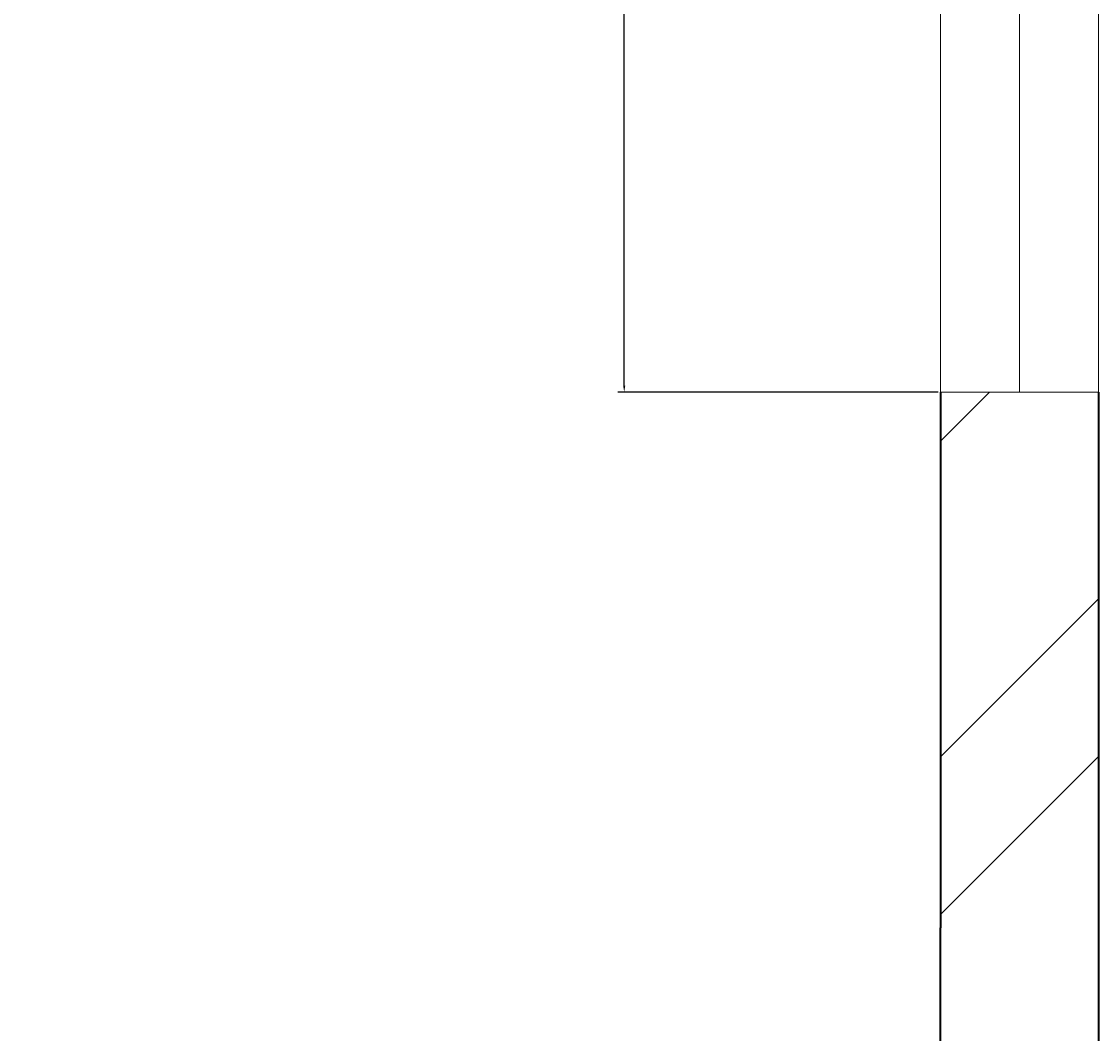
# Model space of a CAD drawing. Units: inches. Extents: x 1885 to 2748, y 783 to 2421.
# Tile 103 of 117: x 2588 to 2618, y 1879 to 1907. Entities that reach past the tile are written whole.
import ezdxf

# ---------------------------------------------------------------- set-up
doc = ezdxf.new("R2010")
doc.units = ezdxf.units.IN
for name, color, linetype, lineweight in [('A-ANNO-DIMS', 2, 'Continuous', 18), ('A-GLAZ', 181, 'Continuous', 18), ('A-WALL', 7, 'Continuous', 35)]:
    doc.layers.add(name, color=color, linetype=linetype, lineweight=lineweight)
doc.layers.add('A-WALL-PATT', color=85, linetype='Continuous', lineweight=13, true_color=0x58ba48)
doc.styles.get("Standard").update_dxf_attribs({"font": 'arial.ttf'})
doc.dimstyles.get("Standard").update_dxf_attribs({"dimtxt": 0.18, "dimasz": 0.18, "dimexe": 0.18, "dimexo": 0.0625, "dimgap": 0.09, "dimtad": 0, "dimtih": 1, "dimtoh": 1, "dimdec": 4, "dimzin": 0, "dimdsep": 46, "dimtxsty": 'Standard', "dimcen": 0.09, "dimadec": 0, "dimazin": 0, "dimtfac": 1, "dimtdec": 4, "dimtofl": 0, "dimtmove": 0, "dimatfit": 3, "dimfxl": 1, "dimtolj": 1, "dimtzin": 0, "dimarcsym": 0})

# ---------------------------------------------------------------- blocks, each defined once
blk = doc.blocks.new('WIN-60-ALT')
for p, q in [((0.004, 59.998), (0.004, -0.002)), ((2.254, 59.998), (2.254, -0.002)), ((4.504, -0.002), (4.504, 59.998)), ((4.504, -0.002), (0.004, -0.002)), ((2.254, -0.002), (4.504, -0.002))]:
    blk.add_line(p, q)
blk = doc.blocks.new('*D17')
at = {"layer": 'A-ANNO-DIMS', "color": 0, "lineweight": -2, "transparency": 16777216}
for p, q in [((2613.711, 1956.755), (2604.594, 1956.755)), ((2604.774, 1956.575), (2604.774, 1926.938)), ((2604.774, 1896.935), (2604.774, 1926.572)), ((2613.711, 1896.755), (2604.594, 1896.755))]:
    blk.add_line(p, q, dxfattribs=at)
at = {"layer": 'A-ANNO-DIMS', "color": 0, "transparency": 16777216}
for points in [[(2604.744, 1956.575), (2604.804, 1956.575), (2604.774, 1956.755)], [(2604.744, 1896.935), (2604.804, 1896.935), (2604.774, 1896.755)]]:
    blk.add_solid(points, dxfattribs=at)
at = {"layer": 'Defpoints', "color": 0, "transparency": 16777216}
for p in [(2604.774, 1956.755), (2613.774, 1956.755), (2613.774, 1896.755)]:
    blk.add_point(p, dxfattribs=at)
at = {"layer": 'A-ANNO-DIMS', "color": 0, "transparency": 16777216, "insert": (2604.774, 1926.755), "char_height": 0.18, "attachment_point": 5}
blk.add_mtext('\\A1;ALT. WINDOW 60 TYP.', dxfattribs=at)

msp = doc.modelspace()

# ---------------------------------------------------------------- hatches: boundary and pattern name
at = {"layer": 'A-WALL-PATT'}
h = msp.add_hatch(dxfattribs=at)
h.set_pattern_fill('ANSI32', color=256)
h.paths.add_polyline_path([(2007.772, 2318.006), (1980.774, 2318.006), (1980.774, 2281.215), (1985.274, 2281.215), (1985.274, 2313.506), (2007.772, 2313.506), (2007.772, 2315.756)])
h.paths.add_polyline_path([(2094.324, 2318.006), (2067.772, 2318.006), (2067.772, 2313.506), (2094.324, 2313.506), (2094.324, 2315.756)])
h.paths.add_polyline_path([(2131.367, 2315.756), (2131.367, 2318.006), (2131.189, 2318.006), (2112.609, 2318.006), (2112.609, 2313.506), (2117.274, 2313.506), (2117.274, 2255.201), (2121.774, 2255.201), (2121.774, 2313.506), (2131.367, 2313.506)])
h.paths.add_polyline_path([(2190.512, 2318.006), (2155.367, 2318.006), (2155.367, 2313.506), (2169.774, 2313.506), (2169.774, 2229.506), (2121.774, 2229.506), (2121.774, 2233.451), (2119.524, 2233.451), (2117.274, 2233.451), (2117.274, 2201.101), (2121.774, 2201.101), (2121.774, 2225.006), (2169.774, 2225.006), (2169.774, 2165.006), (2306.274, 2165.006), (2306.274, 2066.006), (2310.774, 2066.006), (2344.274, 2066.006), (2486.274, 2066.006), (2486.274, 1886.006), (2483.02, 1886.006), (2483.02, 1881.506), (2486.274, 1881.506), (2486.274, 1880.678), (2490.774, 1880.678), (2490.774, 2070.506), (2344.274, 2070.506), (2310.774, 2070.506), (2310.774, 2165.006), (2310.774, 2173.636), (2308.524, 2173.636), (2306.274, 2173.636), (2306.274, 2169.506), (2174.274, 2169.506), (2174.274, 2313.506), (2190.512, 2313.506), (2190.512, 2315.756)])
h.paths.add_polyline_path([(1985.274, 2221.215), (1980.774, 2221.215), (1980.774, 2165.006), (1992.774, 2165.006), (1992.774, 2141.927), (1997.274, 2141.927), (1997.274, 2165.006), (2117.274, 2165.006), (2117.274, 2163.126), (2121.774, 2163.126), (2121.774, 2172.734), (2119.524, 2172.734), (2117.274, 2172.734), (2117.274, 2169.506), (1985.274, 2169.506)])
h.paths.add_polyline_path([(1997.274, 2105.927), (1992.774, 2105.927), (1992.774, 2070.506), (2016.774, 2070.506), (2016.774, 2059.123), (2019.024, 2059.123), (2021.274, 2059.123), (2021.274, 2070.506), (2117.274, 2070.506), (2117.274, 2022.506), (2114.423, 2022.506), (2114.423, 2018.006), (2123.627, 2018.006), (2123.627, 2020.256), (2123.627, 2022.506), (2121.774, 2022.506), (2121.774, 2142.587), (2119.524, 2142.587), (2117.274, 2142.587), (2117.274, 2075.006), (1997.274, 2075.006)])
h.paths.add_polyline_path([(2092.029, 2020.256), (2092.029, 2022.506), (2021.274, 2022.506), (2021.274, 2035.123), (2016.774, 2035.123), (2016.774, 2018.006), (2016.774, 1978.784), (2021.274, 1978.784), (2021.274, 2018.006), (2092.029, 2018.006)])
h.paths.add_polyline_path([(2260.938, 2022.506), (2153.105, 2022.506), (2153.105, 2020.256), (2153.105, 2018.006), (2155.274, 2018.006), (2155.274, 1886.006), (2107.629, 1886.006), (2107.629, 1881.506), (2182.911, 1881.506), (2182.911, 1883.756), (2182.911, 1886.006), (2159.774, 1886.006), (2159.774, 2018.006), (2260.938, 2018.006), (2260.938, 2020.256)])
h.paths.add_polyline_path([(2047.629, 1883.756), (2047.629, 1886.006), (2021.274, 1886.006), (2021.274, 1918.784), (2019.024, 1918.784), (2016.774, 1918.784), (2016.774, 1881.506), (2047.629, 1881.506)])
h.paths.add_polyline_path([(2306.361, 1883.756), (2306.361, 1886.006), (2296.274, 1886.006), (2296.274, 1982.006), (2316.535, 1982.006), (2316.535, 1984.256), (2316.535, 1986.506), (2296.274, 1986.506), (2296.274, 2022.506), (2289.276, 2022.506), (2289.276, 2018.006), (2291.774, 2018.006), (2291.774, 1886.006), (2242.911, 1886.006), (2242.911, 1881.506), (2306.361, 1881.506)], flags=17)
h.paths.add_polyline_path([(1985.274, 1843.006), (2021.6, 1843.006), (2021.534, 1845.441), (2021.477, 1847.506), (1980.774, 1847.506), (1980.774, 1809.446), (1985.274, 1809.446)])
h.paths.add_polyline_path([(2131.482, 1845.256), (2131.482, 1847.506), (2081.534, 1847.506), (2081.534, 1843.006), (2117.274, 1843.006), (2117.274, 1784.147), (2119.524, 1784.147), (2121.774, 1784.147), (2121.774, 1843.006), (2131.482, 1843.006)])
h.paths.add_polyline_path([(2203.886, 1847.506), (2155.482, 1847.506), (2155.482, 1843.006), (2169.774, 1843.006), (2169.774, 1759.006), (2121.774, 1759.006), (2121.774, 1761.457), (2117.274, 1761.457), (2117.274, 1730.429), (2121.774, 1730.429), (2121.774, 1754.506), (2177.421, 1754.506), (2177.421, 1756.756), (2177.421, 1759.006), (2174.274, 1759.006), (2174.274, 1843.006), (2203.886, 1843.006)])
h.paths.add_polyline_path([(2335.554, 1845.256), (2335.554, 1847.506), (2239.886, 1847.506), (2239.886, 1843.006), (2306.274, 1843.006), (2306.274, 1759.006), (2199.486, 1759.006), (2199.486, 1754.506), (2310.774, 1754.506), (2310.774, 1843.006), (2335.554, 1843.006)])
h.paths.add_polyline_path([(2348.774, 2022.506), (2344.274, 2022.506), (2344.274, 1986.506), (2341.681, 1986.506), (2341.681, 1982.006), (2344.274, 1982.006), (2344.274, 1886.006), (2330.361, 1886.006), (2330.361, 1881.506), (2361.627, 1881.506), (2361.627, 1883.756), (2361.627, 1886.006), (2348.774, 1886.006)], flags=17)
h.paths.add_polyline_path([(2283.251, 2315.756), (2283.251, 2318.006), (2238.512, 2318.006), (2238.512, 2313.506), (2283.251, 2313.506)], flags=17)
h.paths.add_polyline_path([(2363.274, 2348.006), (2388.677, 2348.006), (2388.677, 2350.256), (2388.677, 2352.506), (2358.774, 2352.506), (2358.774, 2348.006), (2358.774, 2318.006), (2344.481, 2318.006), (2344.481, 2313.506), (2358.774, 2313.506), (2358.774, 2229.506), (2310.774, 2229.506), (2310.774, 2231.952), (2306.274, 2231.952), (2306.274, 2205.611), (2310.774, 2205.611), (2310.774, 2225.006), (2358.774, 2225.006), (2358.774, 2211.506), (2452.329, 2211.506), (2452.329, 2213.756), (2452.329, 2216.006), (2363.274, 2216.006), (2363.274, 2318.006)])
h.paths.add_polyline_path([(2310.774, 2313.506), (2320.481, 2313.506), (2320.481, 2315.756), (2320.481, 2318.006), (2302.728, 2318.006), (2302.728, 2313.506), (2306.274, 2313.506), (2306.274, 2251.076), (2310.774, 2251.076)], flags=17)
h.paths.add_polyline_path([(2490.774, 2352.506), (2486.274, 2352.506), (2448.677, 2352.506), (2448.677, 2348.006), (2486.274, 2348.006), (2486.274, 2318.006), (2486.274, 2216.006), (2481.78, 2216.006), (2481.78, 2211.506), (2486.274, 2211.506), (2486.274, 2165.006), (2493.289, 2165.006), (2493.289, 2167.256), (2493.289, 2169.506), (2490.774, 2169.506), (2490.774, 2313.506), (2494.429, 2313.506), (2494.429, 2318.006), (2490.774, 2318.006)])
h.paths.add_polyline_path([(2534.653, 2318.006), (2515.691, 2318.006), (2515.691, 2313.506), (2534.653, 2313.506), (2534.653, 2315.756)])
h.paths.add_polyline_path([(2618.274, 2318.006), (2594.653, 2318.006), (2594.653, 2313.506), (2613.774, 2313.506), (2613.774, 2281.706), (2618.274, 2281.706)])
h.paths.add_polyline_path([(2618.274, 2221.706), (2613.774, 2221.706), (2613.774, 2169.506), (2554.019, 2169.506), (2554.019, 2165.006), (2613.774, 2165.006), (2613.774, 2152.878), (2618.274, 2152.878)])
h.paths.add_polyline_path([(2618.274, 2128.878), (2616.024, 2128.878), (2613.774, 2128.878), (2613.774, 2117.006), (2529.774, 2117.006), (2529.774, 2165.006), (2532.848, 2165.006), (2532.848, 2169.506), (2522.867, 2169.506), (2522.867, 2165.006), (2525.274, 2165.006), (2525.274, 2117.006), (2525.274, 2112.506), (2525.274, 2108.576), (2529.774, 2108.576), (2529.774, 2112.506), (2613.774, 2112.506), (2613.774, 2080.19), (2618.274, 2080.19)])
h.paths.add_polyline_path([(2618.274, 2044.19), (2616.024, 2044.19), (2613.774, 2044.19), (2613.774, 2015.506), (2529.774, 2015.506), (2529.774, 2088.582), (2527.524, 2088.582), (2525.274, 2088.582), (2525.274, 2011.006), (2613.774, 2011.006), (2613.774, 1956.755), (2618.274, 1956.755)])
h.paths.add_polyline_path([(2618.274, 1881.506), (2618.274, 1896.755), (2613.774, 1896.755), (2613.774, 1881.506), (2613.774, 1847.506), (2592.715, 1847.506), (2592.715, 1843.006), (2613.774, 1843.006), (2613.774, 1765.006), (2613.774, 1760.506), (2609.621, 1760.506), (2609.621, 1756.006), (2613.774, 1756.006), (2613.774, 1660.006), (2608.544, 1660.006), (2608.544, 1655.506), (2613.774, 1655.506), (2613.774, 1508.158), (2618.274, 1508.158)])
h.paths.add_polyline_path([(2565.774, 1843.006), (2568.997, 1843.006), (2568.997, 1847.506), (2490.774, 1847.506), (2490.774, 1849.7), (2488.524, 1849.7), (2486.274, 1849.7), (2486.274, 1847.506), (2477.274, 1847.506), (2477.274, 1838.506), (2477.274, 1821.493), (2486.274, 1821.493), (2486.274, 1838.506), (2561.274, 1838.506), (2561.274, 1765.006), (2486.274, 1765.006), (2486.274, 1786.157), (2477.274, 1786.157), (2477.274, 1765.006), (2477.274, 1756.006), (2486.274, 1756.006), (2565.774, 1756.006), (2585.621, 1756.006), (2585.621, 1758.256), (2585.621, 1760.506), (2565.774, 1760.506), (2565.774, 1765.006)])
h.paths.add_polyline_path([(2486.274, 1651.006), (2561.274, 1651.006), (2561.274, 1567.006), (2486.274, 1567.006), (2486.274, 1591.321), (2477.274, 1591.321), (2477.274, 1567.006), (2477.274, 1558.006), (2477.274, 1555.439), (2481.774, 1555.439), (2481.774, 1558.006), (2568.653, 1558.006), (2568.653, 1560.256), (2568.653, 1562.506), (2565.774, 1562.506), (2565.774, 1655.506), (2584.544, 1655.506), (2584.544, 1657.756), (2584.544, 1660.006), (2565.774, 1660.006), (2486.274, 1660.006), (2477.274, 1660.006), (2477.274, 1651.006), (2477.274, 1632.989), (2486.274, 1632.989)])
h.paths.add_polyline_path([(2449.967, 1883.756), (2449.967, 1886.006), (2421.627, 1886.006), (2421.627, 1881.506), (2449.967, 1881.506)], flags=17)
h.paths.add_polyline_path([(2447.274, 1847.506), (2395.554, 1847.506), (2395.554, 1843.006), (2442.774, 1843.006), (2442.774, 1809.27), (2447.274, 1809.27)])
h.paths.add_polyline_path([(1985.274, 1749.446), (1980.774, 1749.446), (1980.774, 1694.504), (1985.274, 1694.504), (1985.274, 1694.506), (1986.897, 1694.506), (1986.897, 1697.78), (1986.897, 1699.006), (1985.274, 1699.006)])
h.paths.add_polyline_path([(2152.774, 1699.006), (2121.774, 1699.006), (2121.774, 1703.668), (2119.524, 1703.668), (2117.274, 1703.668), (2117.274, 1699.006), (2009.219, 1699.006), (2009.219, 1694.506), (2148.274, 1694.506), (2148.274, 1692.631), (2152.774, 1692.631)])
h.paths.add_polyline_path([(2016.274, 1694.506), (2011.774, 1694.506), (2011.774, 1558.006), (2040.806, 1558.006), (2040.806, 1560.256), (2040.806, 1562.506), (2016.274, 1562.506)])
h.paths.add_polyline_path([(2152.774, 1663.017), (2150.524, 1663.017), (2148.274, 1663.017), (2148.274, 1562.506), (2100.806, 1562.506), (2100.806, 1558.006), (2165.119, 1558.006), (2165.119, 1560.256), (2165.119, 1562.506), (2152.774, 1562.506), (2152.774, 1610.506), (2224.774, 1610.506), (2224.774, 1607.99), (2229.274, 1607.99), (2229.274, 1615.006), (2152.774, 1615.006)])
h.paths.add_polyline_path([(2238.613, 1560.256), (2238.613, 1562.506), (2229.274, 1562.506), (2229.274, 1588.756), (2227.024, 1588.763), (2224.774, 1588.771), (2224.774, 1562.506), (2189.119, 1562.506), (2189.119, 1558.006), (2238.613, 1558.006)])
h.paths.add_polyline_path([(2336.024, 1560.256), (2336.024, 1562.506), (2310.774, 1562.506), (2310.774, 1656.347), (2308.524, 1656.347), (2306.274, 1656.347), (2306.274, 1562.506), (2286.613, 1562.506), (2286.613, 1558.006), (2336.024, 1558.006)])
h.paths.add_polyline_path([(2447.274, 1690.968), (2445.024, 1690.968), (2442.774, 1690.968), (2442.774, 1687.006), (2306.274, 1687.006), (2306.274, 1680.75), (2310.774, 1680.75), (2310.774, 1682.506), (2442.774, 1682.506), (2442.774, 1562.506), (2396.024, 1562.506), (2396.024, 1558.006), (2447.274, 1558.006)])
h.paths.add_polyline_path([(2447.274, 1749.27), (2445.024, 1749.27), (2442.774, 1749.27), (2442.774, 1717.232), (2447.274, 1717.232)])
h.paths.add_polyline_path([(2044.674, 1521.756), (2044.674, 1524.006), (2007.274, 1524.006), (2007.274, 1503.49), (2009.524, 1503.49), (2011.774, 1503.49), (2011.774, 1519.506), (2044.674, 1519.506)])
h.paths.add_polyline_path([(2177.969, 1521.756), (2177.969, 1524.006), (2104.674, 1524.006), (2104.674, 1519.506), (2145.774, 1519.506), (2145.774, 1387.506), (2143.37, 1387.506), (2143.37, 1383.006), (2251.585, 1383.006), (2251.585, 1385.256), (2251.585, 1387.506), (2150.274, 1387.506), (2150.274, 1519.506), (2177.969, 1519.506)])
h.paths.add_polyline_path([(2298.704, 1524.006), (2237.969, 1524.006), (2237.969, 1519.506), (2282.274, 1519.506), (2282.274, 1387.506), (2279.683, 1387.506), (2279.683, 1383.006), (2286.774, 1383.006), (2286.774, 1419.006), (2312.451, 1419.006), (2312.451, 1421.256), (2312.451, 1423.506), (2286.774, 1423.506), (2286.774, 1519.506), (2298.704, 1519.506), (2298.704, 1521.722)], flags=17)
h.paths.add_polyline_path([(2361.897, 1521.756), (2361.897, 1524.006), (2322.704, 1524.006), (2322.704, 1519.506), (2334.774, 1519.506), (2334.774, 1423.506), (2331.93, 1423.506), (2331.93, 1419.006), (2334.774, 1419.006), (2334.774, 1387.506), (2334.774, 1383.228), (2339.274, 1383.228), (2339.274, 1387.506), (2339.274, 1519.506), (2361.897, 1519.506)], flags=17)
h.paths.add_polyline_path([(2447.274, 1521.756), (2447.274, 1524.006), (2421.897, 1524.006), (2421.897, 1519.506), (2447.274, 1519.506)], flags=17)
h.paths.add_polyline_path([(2481.774, 1529.6), (2479.524, 1529.6), (2477.274, 1529.6), (2477.274, 1524.006), (2474.489, 1524.006), (2474.489, 1519.506), (2477.274, 1519.506), (2477.274, 1334.506), (2296.774, 1334.506), (2296.774, 1240.506), (2160.274, 1240.506), (2160.274, 1180.506), (2112.274, 1180.506), (2112.274, 1207.692), (2110.024, 1207.692), (2107.774, 1207.692), (2107.774, 1171.609), (2112.274, 1171.609), (2112.274, 1176.006), (2160.274, 1176.006), (2160.274, 1092.006), (2144.221, 1092.006), (2144.221, 1087.506), (2189.497, 1087.506), (2189.497, 1089.756), (2189.497, 1092.006), (2164.774, 1092.006), (2164.774, 1236.006), (2296.774, 1236.006), (2296.774, 1231.912), (2301.274, 1231.912), (2301.274, 1330.006), (2481.774, 1330.006), (2481.774, 1387.506)])
h.paths.add_polyline_path([(2618.274, 1448.158), (2613.774, 1448.158), (2613.774, 1382.506), (2529.774, 1382.506), (2525.274, 1382.506), (2525.274, 1307.062), (2529.774, 1307.062), (2529.774, 1378.006), (2613.774, 1378.006), (2613.774, 1354.988), (2618.274, 1354.988)])
h.paths.add_polyline_path([(2618.274, 1318.988), (2613.774, 1318.988), (2613.774, 1281.006), (2529.774, 1281.006), (2529.774, 1283.786), (2527.524, 1283.786), (2525.274, 1283.786), (2525.274, 1228.506), (2516.794, 1228.506), (2516.794, 1224.006), (2533.484, 1224.006), (2533.484, 1226.256), (2533.484, 1228.506), (2529.774, 1228.506), (2529.774, 1276.506), (2613.774, 1276.506), (2613.774, 1266.02), (2618.274, 1266.02)])
h.paths.add_polyline_path([(2618.274, 1134.964), (2613.774, 1134.964), (2613.774, 1092.006), (2594.545, 1092.006), (2594.545, 1087.506), (2618.274, 1087.506)])
h.paths.add_polyline_path([(2534.545, 1092.006), (2509.765, 1092.006), (2509.765, 1087.506), (2534.545, 1087.506), (2534.545, 1089.756)])
h.paths.add_polyline_path([(2481.274, 1224.006), (2484.117, 1224.006), (2484.117, 1226.256), (2484.117, 1228.506), (2476.774, 1228.506), (2476.774, 1198.506), (2471.61, 1198.506), (2471.61, 1194.006), (2476.774, 1194.006), (2476.774, 1062.006), (2436.894, 1062.006), (2436.894, 1057.506), (2476.774, 1057.506), (2481.274, 1057.506), (2481.274, 1062.006), (2481.274, 1087.506), (2485.354, 1087.506), (2485.354, 1089.756), (2485.354, 1092.006), (2481.274, 1092.006), (2481.274, 1117.506)])
h.paths.add_polyline_path([(2439.898, 1198.506), (2349.274, 1198.506), (2349.274, 1194.006), (2349.274, 1180.506), (2301.274, 1180.506), (2301.274, 1201.896), (2299.024, 1201.896), (2296.774, 1201.896), (2296.774, 1172.335), (2299.024, 1172.335), (2301.274, 1172.335), (2301.274, 1176.006), (2349.274, 1176.006), (2349.274, 1092.006), (2334.452, 1092.006), (2334.452, 1087.506), (2349.274, 1087.506), (2349.274, 1057.506), (2353.774, 1057.506), (2376.894, 1057.506), (2376.894, 1059.756), (2376.894, 1062.006), (2353.774, 1062.006), (2353.774, 1087.506), (2353.774, 1180.506), (2353.774, 1194.006), (2439.898, 1194.006), (2439.898, 1196.256)])
h.paths.add_polyline_path([(2270.596, 1089.756), (2270.596, 1092.006), (2249.497, 1092.006), (2249.497, 1087.506), (2270.596, 1087.506)], flags=17)
h.paths.add_polyline_path([(2310.452, 1092.006), (2301.274, 1092.006), (2301.274, 1153.292), (2296.774, 1153.292), (2296.774, 1092.006), (2293.786, 1092.006), (2293.786, 1087.506), (2310.452, 1087.506), (2310.452, 1089.756)], flags=17)
h.paths.add_polyline_path([(2112.274, 1150.328), (2110.024, 1150.328), (2107.774, 1150.328), (2107.774, 1092.006), (2104.465, 1092.006), (2104.465, 1087.506), (2120.221, 1087.506), (2120.221, 1089.756), (2120.221, 1092.006), (2112.274, 1092.006)])
h.paths.add_polyline_path([(2082.172, 1092.006), (2058.144, 1092.006), (2058.144, 1087.506), (2082.172, 1087.506), (2082.172, 1089.756)])
h.paths.add_polyline_path([(1975.774, 1145.638), (1971.274, 1145.638), (1971.274, 1087.506), (1980.774, 1087.506), (1998.144, 1087.506), (1998.144, 1089.756), (1998.144, 1092.006), (1985.274, 1092.006), (1975.774, 1092.006)])
h.paths.add_polyline_path([(2112.274, 1244.385), (2110.024, 1244.385), (2107.774, 1244.385), (2107.774, 1240.506), (1992.274, 1240.506), (1992.274, 1271.008), (1987.774, 1271.008), (1987.774, 1240.506), (1980.774, 1240.506), (1975.774, 1240.506), (1971.274, 1240.506), (1971.274, 1205.638), (1975.774, 1205.638), (1975.774, 1236.006), (2107.774, 1236.006), (2107.774, 1233.444), (2112.274, 1233.444), (2112.274, 1236.006)])
h.paths.add_polyline_path([(2112.274, 1383.006), (2114.783, 1383.006), (2114.783, 1385.256), (2114.783, 1387.506), (2102.476, 1387.506), (2102.476, 1383.006), (2107.774, 1383.006), (2107.774, 1335.006), (2011.774, 1335.006), (2011.774, 1349.939), (2007.274, 1349.939), (2007.274, 1335.006), (1987.774, 1335.006), (1987.774, 1330.506), (1987.774, 1307.008), (1992.274, 1307.008), (1992.274, 1330.506), (2007.274, 1330.506), (2107.774, 1330.506), (2107.774, 1264.711), (2112.274, 1264.711)])
h.paths.add_polyline_path([(2077.857, 1387.506), (2011.774, 1387.506), (2011.774, 1390.036), (2009.524, 1390.036), (2007.274, 1390.036), (2007.274, 1373.939), (2011.774, 1373.939), (2011.774, 1383.006), (2077.857, 1383.006)])
h.paths.add_polyline_path([(2011.774, 1443.49), (2007.274, 1443.49), (2007.274, 1410.248), (2011.774, 1410.248)])

# ---------------------------------------------------------------- linework, layer by layer
at = {"layer": 'A-WALL'}
for p, q in [((2613.774, 1896.755), (2613.774, 1881.506)), ((2618.274, 1896.755), (2618.274, 1881.506)), ((2613.774, 1847.506), (2613.774, 1881.506)), ((2618.274, 1881.506), (2618.274, 1508.158))]:
    msp.add_line(p, q, dxfattribs=at)

# ---------------------------------------------------------------- block references
at = {"layer": 'A-GLAZ'}
msp.add_blockref('WIN-60-ALT', (2613.77, 1896.757), dxfattribs=at)

# ---------------------------------------------------------------- dimensions: what is measured, and where the dimension line sits
at = {"layer": 'A-ANNO-DIMS'}
dim = msp.add_linear_dim(base=(2604.774, 1956.755), p1=(2613.774, 1896.755), p2=(2613.774, 1956.755), angle=90, text='ALT. WINDOW <> TYP.', dimstyle='Standard', override={"dimdec": 0, "dimlfac": 1, "dimrnd": 0, "dimzin": 0, "dimdsep": 46, "dimlunit": 2}, dxfattribs=at)
dim.commit()
dim.dimension.update_dxf_attribs({"geometry": '*D17', "text_midpoint": (2604.774, 1926.755)})

doc.saveas('drawing.dxf')
